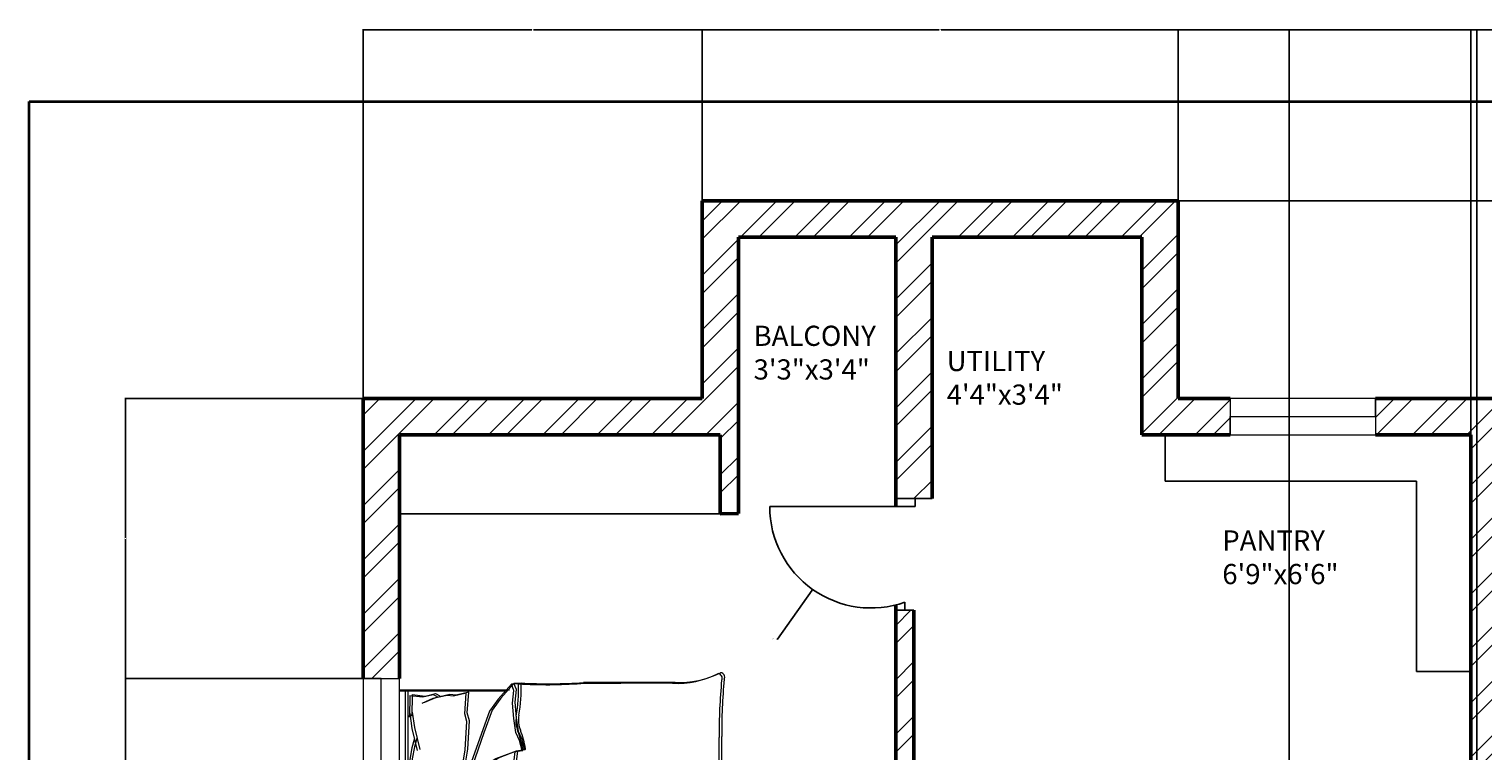
# Model space of a CAD drawing. Units: inches. Extents: x 1896 to 2572, y 1528 to 2474.
# Tile 8 of 10: x 1896 to 2256, y 2295 to 2474. Entities that reach past the tile are written whole.
import ezdxf

# ---------------------------------------------------------------- set-up
doc = ezdxf.new("R2010")
doc.units = ezdxf.units.IN
for name, color, linetype, lineweight in [('A-ANNO-DIMS', 2, 'Continuous', 18), ('A-ANNO-TTLB', 7, 'Continuous', 35), ('A-AREA-IDEN', 7, 'Continuous', 18), ('A-DOOR', 11, 'Continuous', 25), ('A-FLOR-CASE', 7, 'Continuous', 25), ('A-FURN', 8, 'Continuous', 18), ('A-GLAZ', 131, 'Continuous', 20), ('A-WALL', 7, 'Continuous', 50)]:
    doc.layers.add(name, color=color, linetype=linetype, lineweight=lineweight)
doc.layers.add('A-WALL-PATT', color=215, linetype='Continuous', lineweight=13, true_color=0xa953a0)
doc.styles.get("Standard").update_dxf_attribs({"font": 'arial.ttf'})
doc.dimstyles.get("Standard").update_dxf_attribs({"dimtxt": 0.18, "dimasz": 0.18, "dimexe": 0.18, "dimexo": 0.0625, "dimgap": 0.09, "dimtad": 0, "dimtih": 1, "dimtoh": 1, "dimdec": 4, "dimzin": 0, "dimdsep": 46, "dimtxsty": 'Standard', "dimcen": 0.09, "dimadec": 0, "dimazin": 0, "dimtfac": 1, "dimtdec": 4, "dimtofl": 0, "dimtmove": 0, "dimatfit": 3, "dimfxl": 1, "dimtolj": 1, "dimtzin": 0, "dimarcsym": 0})

# ---------------------------------------------------------------- blocks, each defined once
blk = doc.blocks.new('BED-DOUBLE')
for p, q in [((3.47, 63.33), (3.47, 81.44)), ((3.47, 63.33), (3.47, 81.44)), ((3.47, 81.44), (51.49, 81.44)), ((3.47, 79.91), (51.27, 79.91)), ((3.47, 79.91), (51.26, 79.91)), ((3.7, 62.69), (3.7, 80.8)), ((3.7, 62.69), (3.7, 80.8)), ((3.7, 79.27), (51.49, 79.27)), ((3.7, 79.27), (51.49, 79.27)), ((24.54, 78.99), (25.98, 79.57)), ((24.54, 78.99), (25.98, 79.57)), ((25.98, 79.57), (26.56, 74.22)), ((25.98, 79.57), (26.56, 74.22)), ((51.26, 81.44), (51.26, 54.83)), ((51.27, 81.44), (51.27, 54.83)), ((51.49, 81.44), (51.49, 80.8)), ((51.49, 80.8), (51.49, 54.19)), ((51.49, 80.8), (51.49, 54.19)), ((3.89, 78.13), (4.47, 74.95)), ((3.89, 78.13), (4.47, 74.95)), ((3.9, 78.11), (8.18, 78.43)), ((3.9, 78.11), (8.18, 78.43)), ((4.12, 77.49), (4.7, 74.31)), ((4.12, 77.49), (4.7, 74.31)), ((4.13, 77.47), (8.41, 77.8)), ((4.13, 77.47), (8.41, 77.8)), ((8.18, 78.43), (8.28, 78.42)), ((8.18, 78.43), (8.28, 78.42)), ((8.28, 78.42), (12.11, 78.13)), ((8.28, 78.42), (12.11, 78.13)), ((8.41, 77.8), (8.51, 77.78)), ((8.41, 77.8), (8.51, 77.78)), ((8.51, 77.78), (12.34, 77.49)), ((8.51, 77.78), (12.34, 77.49)), ((12.11, 78.13), (17.6, 77.12)), ((12.11, 78.13), (17.6, 77.12)), ((12.34, 77.49), (17.83, 76.48)), ((12.34, 77.49), (17.83, 76.48)), ((14.85, 77.69), (16.88, 78.42)), ((14.85, 77.69), (16.88, 78.42)), ((15.08, 77.05), (17.11, 77.78)), ((15.08, 77.05), (17.11, 77.78)), ((16.88, 78.42), (19.77, 79.14)), ((16.88, 78.42), (19.77, 79.14)), ((17.11, 77.78), (20, 78.5)), ((17.11, 77.78), (20, 78.5)), ((19.77, 79.14), (20.09, 79.14)), ((19.77, 79.14), (20.09, 79.14)), ((20, 78.5), (20.32, 78.5)), ((20, 78.5), (20.32, 78.5)), ((20.09, 79.14), (24.54, 78.99)), ((20.09, 79.14), (24.54, 78.99)), ((20.32, 78.5), (24.77, 78.36)), ((20.32, 78.5), (24.76, 78.36)), ((24.76, 78.36), (26.21, 78.93)), ((24.77, 78.36), (26.21, 78.93)), ((26.21, 78.93), (26.79, 73.58)), ((26.21, 78.93), (26.79, 73.58)), ((27.98, 78.95), (27.73, 73.58)), ((27.98, 78.95), (27.73, 73.58)), ((28.21, 78.31), (27.96, 72.94)), ((28.2, 78.31), (27.96, 72.94)), ((29.46, 78.46), (27.98, 78.95)), ((29.46, 78.46), (27.98, 78.95)), ((29.68, 77.83), (28.2, 78.31)), ((29.68, 77.83), (28.21, 78.31)), ((33.88, 78.89), (29.46, 78.46)), ((33.88, 78.89), (29.46, 78.46)), ((34.11, 78.25), (29.68, 77.83)), ((34.11, 78.25), (29.68, 77.83)), ((34.2, 78.91), (33.88, 78.89)), ((34.2, 78.91), (33.88, 78.89)), ((34.43, 78.27), (34.11, 78.25)), ((34.43, 78.27), (34.11, 78.25)), ((37.14, 78.37), (34.2, 78.91)), ((37.13, 78.37), (34.2, 78.91)), ((37.36, 77.73), (34.43, 78.27)), ((37.36, 77.73), (34.43, 78.27)), ((41.91, 78.37), (36.49, 77.02)), ((41.91, 78.37), (36.49, 77.02)), ((42.14, 77.73), (36.72, 76.38)), ((42.14, 77.73), (36.72, 76.38)), ((39.2, 77.77), (37.13, 78.37)), ((39.2, 77.77), (37.14, 78.37)), ((39.43, 77.13), (37.36, 77.73)), ((39.43, 77.13), (37.36, 77.73)), ((45.71, 78.9), (41.91, 78.37)), ((45.71, 78.9), (41.91, 78.37)), ((45.94, 78.26), (42.14, 77.73)), ((45.94, 78.26), (42.14, 77.73)), ((50.11, 78.89), (44.71, 78.98)), ((44.71, 78.98), (45.71, 78.9)), ((50.11, 78.89), (44.71, 78.98)), ((44.71, 78.98), (45.71, 78.9)), ((50.34, 78.25), (44.94, 78.34)), ((44.94, 78.34), (45.94, 78.26)), ((50.34, 78.25), (44.94, 78.34)), ((44.94, 78.34), (45.94, 78.26)), ((49.31, 73.19), (48.13, 75.87)), ((49.31, 73.19), (48.13, 75.87)), ((50.11, 78.89), (49.73, 75.68)), ((50.11, 78.89), (49.73, 75.68)), ((49.73, 75.68), (50.33, 73.11)), ((49.73, 75.68), (50.33, 73.11)), ((50.34, 78.25), (49.96, 75.04)), ((50.34, 78.25), (49.96, 75.04)), ((4.47, 74.95), (4.04, 72.34)), ((4.47, 74.95), (4.04, 72.34)), ((4.04, 72.34), (4.62, 71.33)), ((4.04, 72.34), (4.62, 71.33)), ((4.7, 74.31), (4.27, 71.7)), ((4.7, 74.31), (4.27, 71.7)), ((4.47, 68.87), (5.05, 72.49)), ((4.47, 68.87), (5.05, 72.49)), ((5.05, 72.49), (6.06, 75.24)), ((5.05, 72.49), (6.06, 75.24)), ((5.28, 71.85), (6.29, 74.6)), ((5.28, 71.85), (6.29, 74.6)), ((26.56, 74.22), (27.14, 71.04)), ((26.56, 74.22), (27.14, 71.04)), ((26.79, 73.58), (27.37, 70.4)), ((26.79, 73.58), (27.37, 70.4)), ((27.73, 73.58), (27.35, 70.37)), ((27.73, 73.58), (27.35, 70.37)), ((27.96, 72.94), (27.58, 69.73)), ((27.96, 72.94), (27.58, 69.73)), ((49.54, 72.55), (48.36, 75.23)), ((49.54, 72.55), (48.36, 75.23)), ((50.11, 69.61), (49.31, 73.19)), ((50.11, 69.61), (49.31, 73.19)), ((50.34, 68.98), (49.54, 72.55)), ((50.34, 68.98), (49.54, 72.55)), ((50.33, 73.11), (49.81, 72.06)), ((50.33, 73.11), (49.81, 72.06)), ((49.96, 75.04), (50.56, 72.47)), ((49.96, 75.04), (50.56, 72.47)), ((50.56, 72.47), (50.04, 71.42)), ((50.56, 72.47), (50.04, 71.42)), ((4.27, 71.7), (4.85, 70.69)), ((4.27, 71.7), (4.85, 70.69)), ((4.76, 67.28), (4.47, 68.87)), ((4.76, 67.28), (4.47, 68.87)), ((4.7, 68.23), (5.28, 71.85)), ((4.7, 68.23), (5.28, 71.85)), ((27.14, 69.74), (26.56, 67.86)), ((27.14, 69.74), (26.56, 67.86)), ((27.37, 69.1), (26.79, 67.22)), ((27.37, 69.1), (26.79, 67.22)), ((27.14, 71.04), (27.14, 69.74)), ((27.14, 71.04), (27.14, 69.74)), ((27.35, 70.37), (27.44, 69.07)), ((27.35, 70.37), (27.44, 69.07)), ((27.37, 70.4), (27.37, 69.1)), ((27.37, 70.4), (27.37, 69.1)), ((27.44, 69.07), (28.13, 67.23)), ((27.44, 69.07), (28.13, 67.23)), ((27.58, 69.73), (27.66, 68.43)), ((27.58, 69.73), (27.66, 68.43)), ((49.92, 68.01), (50.11, 69.61)), ((49.92, 68.01), (50.11, 69.61)), ((50.15, 67.37), (50.34, 68.98)), ((50.15, 67.37), (50.34, 68.98)), ((4.18, 64.1), (4.76, 67.28)), ((4.18, 64.1), (4.76, 67.28)), ((4.41, 63.46), (4.99, 66.64)), ((4.41, 63.46), (4.99, 66.64)), ((4.99, 66.64), (4.7, 68.23)), ((4.99, 66.64), (4.7, 68.23)), ((6.38, 65.81), (10.41, 65.15)), ((6.38, 65.81), (10.41, 65.15)), ((6.61, 65.18), (10.64, 64.51)), ((6.61, 65.18), (10.64, 64.51)), ((10.41, 65.15), (9.28, 64.83)), ((10.41, 65.15), (9.28, 64.83)), ((10.41, 65.15), (17.42, 64.72)), ((10.41, 65.15), (17.42, 64.72)), ((17.42, 64.72), (19.38, 65.27)), ((17.42, 64.72), (19.38, 65.27)), ((19.38, 65.27), (24.52, 64.87)), ((19.38, 65.27), (24.52, 64.87)), ((24.1, 65.18), (20.96, 66.27)), ((24.1, 65.18), (20.96, 66.27)), ((24.33, 64.54), (21.19, 65.63)), ((24.33, 64.54), (21.19, 65.63)), ((26.56, 65.18), (24.1, 65.18)), ((26.56, 65.18), (24.1, 65.18)), ((26.56, 67.86), (26.56, 65.18)), ((26.56, 67.86), (26.56, 65.18)), ((26.79, 67.22), (26.79, 64.54)), ((26.79, 67.22), (26.79, 64.54)), ((27.66, 68.43), (28.36, 66.59)), ((27.66, 68.43), (28.36, 66.59)), ((28.13, 67.23), (28.3, 64.55)), ((28.13, 67.23), (28.3, 64.55)), ((28.36, 66.59), (28.53, 63.91)), ((28.36, 66.59), (28.53, 63.91)), ((30.75, 64.7), (33.82, 65.99)), ((30.75, 64.7), (33.82, 65.99)), ((30.98, 64.06), (34.05, 65.35)), ((30.98, 64.06), (34.05, 65.35)), ((32.56, 65.81), (36.6, 65.15)), ((32.56, 65.81), (36.6, 65.15)), ((32.79, 65.18), (36.82, 64.51)), ((32.79, 65.18), (36.82, 64.51)), ((36.6, 65.15), (43.61, 64.72)), ((36.6, 65.15), (43.61, 64.72)), ((43.61, 64.72), (45.57, 65.27)), ((43.61, 64.72), (45.57, 65.27)), ((45.57, 65.27), (50.7, 64.87)), ((45.57, 65.27), (50.7, 64.87)), ((50.7, 64.87), (49.92, 68.01)), ((50.7, 64.87), (49.92, 68.01)), ((50.93, 64.23), (50.15, 67.37)), ((50.93, 64.23), (50.15, 67.37)), ((9.28, 64.83), (4.18, 64.1)), ((9.28, 64.83), (4.18, 64.1)), ((9.51, 64.19), (4.41, 63.46)), ((9.51, 64.19), (4.41, 63.46)), ((10.64, 64.51), (9.51, 64.19)), ((10.64, 64.51), (9.51, 64.19)), ((10.64, 64.51), (17.65, 64.08)), ((10.64, 64.51), (17.65, 64.08)), ((17.65, 64.08), (19.61, 64.63)), ((17.65, 64.08), (19.61, 64.63)), ((19.61, 64.63), (24.74, 64.23)), ((19.61, 64.63), (24.74, 64.23)), ((26.79, 64.54), (24.33, 64.54)), ((26.79, 64.54), (24.33, 64.54)), ((28.3, 64.55), (30.75, 64.7)), ((28.3, 64.55), (30.75, 64.7)), ((28.53, 63.91), (30.98, 64.06)), ((28.53, 63.91), (30.98, 64.06)), ((30.26, 64.06), (34.45, 57.57)), ((30.26, 64.06), (34.45, 57.57)), ((30.49, 63.42), (34.68, 56.93)), ((30.49, 63.42), (34.68, 56.93)), ((40.64, 61.13), (32.31, 64.06)), ((40.64, 61.13), (32.31, 64.06)), ((40.87, 60.49), (32.53, 63.42)), ((40.87, 60.49), (32.53, 63.42)), ((36.82, 64.51), (43.83, 64.08)), ((36.82, 64.51), (43.83, 64.08)), ((43.83, 64.08), (45.79, 64.63)), ((43.83, 64.08), (45.79, 64.63)), ((45.79, 64.63), (50.93, 64.23)), ((45.79, 64.63), (50.93, 64.23)), ((46.22, 59.11), (40.64, 61.13)), ((46.22, 59.11), (40.64, 61.13)), ((46.45, 58.48), (40.87, 60.49)), ((46.45, 58.48), (40.87, 60.49)), ((49.16, 56.95), (46.22, 59.11)), ((49.16, 56.95), (46.22, 59.11)), ((49.39, 56.31), (46.45, 58.48)), ((49.39, 56.31), (46.45, 58.48)), ((34.45, 57.57), (36.15, 53.08)), ((34.45, 57.57), (36.15, 53.08)), ((34.68, 56.93), (36.38, 52.44)), ((34.68, 56.93), (36.38, 52.44)), ((52.87, 53.7), (49.16, 56.95)), ((52.87, 53.7), (49.16, 56.95)), ((53.1, 53.06), (49.39, 56.31)), ((53.1, 53.06), (49.39, 56.31)), ((36.15, 53.08), (36.46, 51.07)), ((36.15, 53.08), (36.46, 51.07)), ((36.38, 52.44), (36.69, 50.43)), ((36.38, 52.44), (36.69, 50.43)), ((36.46, 51.07), (38.94, 51.69)), ((36.46, 51.07), (38.94, 51.69)), ((36.69, 50.43), (39.17, 51.05)), ((36.69, 50.43), (39.17, 51.05)), ((38.94, 51.69), (40.95, 52.61)), ((38.94, 51.69), (40.95, 52.61)), ((39.17, 51.05), (41.18, 51.97)), ((39.17, 51.05), (41.18, 51.97)), ((40.95, 52.61), (44.36, 53.08)), ((40.95, 52.61), (44.36, 53.08)), ((41.18, 51.97), (44.59, 52.44)), ((41.18, 51.97), (44.59, 52.44)), ((44.36, 53.08), (48.23, 53.39)), ((44.36, 53.08), (48.23, 53.39)), ((44.59, 52.44), (48.46, 52.75)), ((44.59, 52.44), (48.46, 52.75)), ((48.23, 53.39), (51.33, 53.08)), ((48.23, 53.39), (51.33, 53.08)), ((48.46, 52.75), (51.56, 52.44)), ((48.46, 52.75), (51.56, 52.44)), ((51.33, 53.08), (52.87, 53.7)), ((51.33, 53.08), (52.87, 53.7)), ((51.56, 52.44), (53.1, 53.06)), ((51.56, 52.44), (53.1, 53.06)), ((52.95, 51.95), (52.87, 53.7, 3.87)), ((52.95, 51.95), (52.87, 53.7, 3.87)), ((53.18, 51.31), (53.1, 53.06, 3.87)), ((53.17, 51.31), (53.1, 53.06, 3.87)), ((15.06, 2.2), (39.68, 2.2)), ((15.06, 2.2), (39.68, 2.2)), ((15.29, 1.56), (39.91, 1.56)), ((15.29, 1.56), (39.91, 1.56))]:
    blk.add_line(p, q)
for centre, radius, start, end in [((85.16, 61.35), 83.31, 178.7218, 185.604), ((85.16, 61.35), 83.31, 178.7218, 185.604), ((21.36, -100.61), 164.97, 86.0865, 96.7821), ((21.36, -100.61), 164.97, 86.0865, 96.7821), ((85.39, 60.71), 83.31, 178.7218, 185.604), ((85.39, 60.71), 83.31, 178.7218, 185.604), ((21.59, -101.25), 164.97, 86.0865, 96.7821), ((21.59, -101.25), 164.97, 86.0865, 96.7821), ((17.76, -74.87), 129.02, 81.7845, 96.9006), ((17.76, -74.87), 129.02, 81.7845, 96.9006), ((17.98, -75.51), 129.02, 81.7845, 96.9006), ((17.98, -75.51), 129.02, 81.7845, 96.9006), ((-167.31, 50.27), 170.11, 358.4762, 1.0082), ((-167.31, 50.27), 170.11, 358.4762, 1.0082), ((-167.08, 49.63), 170.11, 358.4762, 1.0082), ((-167.08, 49.63), 170.11, 358.4762, 1.0082), ((36.64, 51), 0.185, 160.2464, 271.1377), ((36.64, 51), 0.185, 160.2464, 271.1377), ((31.15, 79.96), 29.65, 280.6617, 289.8806), ((31.15, 79.96), 29.65, 280.6617, 289.8806), ((31.38, 79.32), 29.65, 280.6617, 289.8806), ((31.38, 79.32), 29.65, 280.6617, 289.8806), ((43.74, 46.38), 6.22, 78.6608, 113.7384), ((43.74, 46.38), 6.22, 78.6608, 113.7384), ((43.97, 45.74), 6.22, 78.6608, 113.7384), ((43.97, 45.74), 6.22, 78.6608, 113.7384), ((51.33, 88.1), 36.18, 259.8763, 272.5657), ((51.33, 88.1), 36.18, 259.8763, 272.5657), ((51.56, 87.46), 36.18, 259.8763, 272.5657), ((51.56, 87.46), 36.18, 259.8763, 272.5657), ((182.27, 45.13), 129.5, 176.9791, 183.8365), ((182.27, 45.13), 129.5, 176.9791, 183.8365), ((182.49, 44.49), 129.5, 176.9791, 183.8365), ((182.49, 44.49), 129.5, 176.9791, 183.8365), ((36.86, 50.36), 0.185, 160.2464, 271.1377), ((36.86, 50.36), 0.185, 160.2464, 271.1377), ((484.82, 30.83), 482.31, 178.2277, 181.7185), ((484.82, 30.83), 482.31, 178.2277, 181.7185), ((485.05, 30.19), 482.31, 178.2277, 181.7185), ((485.05, 30.19), 482.31, 178.2277, 181.7185), ((-4508.74, 13.62), 4561.86, 0.00217, 0.28689), ((-4508.74, 13.62), 4561.86, 0.00217, 0.28689), ((-4508.52, 12.98), 4561.86, 0.00217, 0.28689), ((-4508.52, 12.98), 4561.86, 0.00217, 0.28689), ((-26.9, 16.93), 29.63, 346.0648, 358.9113), ((-26.9, 16.93), 29.63, 346.0648, 358.9113), ((-26.67, 16.29), 29.63, 346.0648, 358.9113), ((-26.67, 16.29), 29.63, 346.0648, 358.9113), ((76.16, 12.78), 23.07, 177.4714, 206.4681), ((76.16, 12.78), 23.07, 177.4714, 206.4681), ((76.39, 12.14), 23.07, 177.4714, 206.4681), ((76.39, 12.14), 23.07, 177.4714, 206.4681), ((-21.66, 11.17), 23.56, 337.9751, 356.652), ((-21.66, 11.17), 23.56, 337.9751, 356.652), ((-21.43, 10.53), 23.56, 337.9751, 356.652), ((-21.43, 10.53), 23.56, 337.9751, 356.652), ((-17.22, 105.16), 106.46, 283.3832, 287.7053), ((-17.22, 105.16), 106.46, 283.3832, 287.7053), ((1.09, 1.73), 1.09, 146.1736, 293.4781), ((1.09, 1.73), 1.09, 146.1736, 293.4781), ((1.32, 1.09), 1.09, 146.1736, 293.4781), ((1.32, 1.09), 1.09, 146.1736, 293.4781), ((21.43, -119.39), 121.76, 92.9958, 99.4091), ((21.43, -119.39), 121.76, 92.9958, 99.4091), ((21.65, -120.03), 121.76, 92.9958, 99.4091), ((21.65, -120.03), 121.76, 92.9958, 99.4091), ((-16.99, 104.52), 106.46, 283.3832, 287.7053), ((-16.99, 104.52), 106.46, 283.3832, 287.7053), ((41.15, -130.83), 133.04, 84.4998, 90.6351), ((41.15, -130.83), 133.04, 84.4998, 90.6351), ((41.38, -131.47), 133.04, 84.4998, 90.6351), ((41.38, -131.47), 133.04, 84.4998, 90.6351), ((54.41, 2.57), 1.1, 242.6588, 356.02), ((54.41, 2.57), 1.1, 242.6588, 356.02), ((54.64, 1.93), 1.1, 242.6588, 356.02), ((54.64, 1.93), 1.1, 242.6588, 356.02)]:
    blk.add_arc(centre, radius, start, end)
blk = doc.blocks.new('WIN-36IN')
for p, q in [((0, 36), (9, 36)), ((0, 0), (0, 36)), ((9, 36), (4.5, 36)), ((4.5, 36), (4.5, 0)), ((9, 36), (9, 0)), ((4.5, 0), (0, 0)), ((0, 0), (9, 0))]:
    blk.add_line(p, q)
blk = doc.blocks.new('WIN-60IN')
for p, q in [((4.5, 60), (0, 60)), ((0, 60), (9, 60)), ((0, 60), (0, 0)), ((4.5, 0), (4.5, 60)), ((9, 0), (9, 60)), ((0, 0), (9, 0)), ((9, 0), (4.5, 0))]:
    blk.add_line(p, q)
blk = doc.blocks.new('*D20')
at = {"layer": 'A-ANNO-DIMS', "color": 0, "lineweight": -2, "transparency": 16777216}
for p, q in [((2180.68, 2431.4), (2511.65, 2431.4)), ((2511.47, 2431.22), (2511.47, 2049.83)), ((2511.47, 1668.08), (2511.47, 2049.47)), ((2452.68, 1667.9), (2511.65, 1667.9))]:
    blk.add_line(p, q, dxfattribs=at)
at = {"layer": 'A-ANNO-DIMS', "color": 0, "transparency": 16777216}
for points in [[(2511.44, 2431.22), (2511.5, 2431.22), (2511.47, 2431.4)], [(2511.44, 1668.08), (2511.5, 1668.08), (2511.47, 1667.9)]]:
    blk.add_solid(points, dxfattribs=at)
at = {"layer": 'Defpoints', "color": 0, "transparency": 16777216}
for p in [(2180.62, 2431.4), (2511.47, 2431.4), (2452.62, 1667.9)]:
    blk.add_point(p, dxfattribs=at)
at = {"layer": 'A-ANNO-DIMS', "color": 0, "transparency": 16777216, "insert": (2511.47, 2049.65), "char_height": 0.18, "attachment_point": 5}
blk.add_mtext('\\A1;763.5', dxfattribs=at)
blk = doc.blocks.new('*D21')
at = {"layer": 'A-ANNO-DIMS', "color": 0, "lineweight": -2, "transparency": 16777216}
for p, q in [((1978.62, 2382.46), (1978.62, 2473.93)), ((1978.8, 2473.75), (2020.4, 2473.75)), ((2062.44, 2473.75), (2020.84, 2473.75)), ((2062.62, 2431.46), (2062.62, 2473.93))]:
    blk.add_line(p, q, dxfattribs=at)
at = {"layer": 'A-ANNO-DIMS', "color": 0, "transparency": 16777216}
for points in [[(1978.8, 2473.78), (1978.8, 2473.72), (1978.62, 2473.75)], [(2062.44, 2473.78), (2062.44, 2473.72), (2062.62, 2473.75)]]:
    blk.add_solid(points, dxfattribs=at)
at = {"layer": 'Defpoints', "color": 0, "transparency": 16777216}
for p in [(2062.62, 2473.75), (2062.62, 2431.4), (1978.62, 2382.4)]:
    blk.add_point(p, dxfattribs=at)
at = {"layer": 'A-ANNO-DIMS', "color": 0, "transparency": 16777216, "insert": (2020.62, 2473.75), "char_height": 0.18, "attachment_point": 5}
blk.add_mtext('\\A1;84', dxfattribs=at)
blk = doc.blocks.new('*D22')
at = {"layer": 'A-ANNO-DIMS', "color": 0, "lineweight": -2, "transparency": 16777216}
for p, q in [((2062.62, 2431.46), (2062.62, 2473.93)), ((2062.8, 2473.75), (2121.34, 2473.75)), ((2180.44, 2473.75), (2121.9, 2473.75)), ((2180.62, 2431.46), (2180.62, 2473.93))]:
    blk.add_line(p, q, dxfattribs=at)
at = {"layer": 'A-ANNO-DIMS', "color": 0, "transparency": 16777216}
for points in [[(2062.8, 2473.78), (2062.8, 2473.72), (2062.62, 2473.75)], [(2180.44, 2473.78), (2180.44, 2473.72), (2180.62, 2473.75)]]:
    blk.add_solid(points, dxfattribs=at)
at = {"layer": 'Defpoints', "color": 0, "transparency": 16777216}
for p in [(2180.62, 2473.75), (2062.62, 2431.4), (2180.62, 2431.4)]:
    blk.add_point(p, dxfattribs=at)
at = {"layer": 'A-ANNO-DIMS', "color": 0, "transparency": 16777216, "insert": (2121.62, 2473.75), "char_height": 0.18, "attachment_point": 5}
blk.add_mtext('\\A1;118', dxfattribs=at)
blk = doc.blocks.new('*D23')
at = {"layer": 'A-ANNO-DIMS', "color": 0, "lineweight": -2, "transparency": 16777216}
for p, q in [((2180.62, 2431.46), (2180.62, 2473.93)), ((2180.8, 2473.75), (2216.55, 2473.75)), ((2252.94, 2473.75), (2217.2, 2473.75)), ((2253.12, 2373.46), (2253.12, 2473.93))]:
    blk.add_line(p, q, dxfattribs=at)
at = {"layer": 'A-ANNO-DIMS', "color": 0, "transparency": 16777216}
for points in [[(2180.8, 2473.78), (2180.8, 2473.72), (2180.62, 2473.75)], [(2252.94, 2473.78), (2252.94, 2473.72), (2253.12, 2473.75)]]:
    blk.add_solid(points, dxfattribs=at)
at = {"layer": 'Defpoints', "color": 0, "transparency": 16777216}
for p in [(2253.12, 2473.75), (2180.62, 2431.4), (2253.12, 2373.4)]:
    blk.add_point(p, dxfattribs=at)
at = {"layer": 'A-ANNO-DIMS', "color": 0, "transparency": 16777216, "insert": (2216.87, 2473.75), "char_height": 0.18, "attachment_point": 5}
blk.add_mtext('\\A1;72.5', dxfattribs=at)
blk = doc.blocks.new('*D24')
at = {"layer": 'A-ANNO-DIMS', "color": 0, "lineweight": -2, "transparency": 16777216}
for p, q in [((2253.12, 2373.46), (2253.12, 2473.93)), ((2253.3, 2473.75), (2352.49, 2473.75)), ((2452.44, 2473.75), (2353.26, 2473.75)), ((2452.62, 2382.46), (2452.62, 2473.93))]:
    blk.add_line(p, q, dxfattribs=at)
at = {"layer": 'A-ANNO-DIMS', "color": 0, "transparency": 16777216}
for points in [[(2253.3, 2473.78), (2253.3, 2473.72), (2253.12, 2473.75)], [(2452.44, 2473.78), (2452.44, 2473.72), (2452.62, 2473.75)]]:
    blk.add_solid(points, dxfattribs=at)
at = {"layer": 'Defpoints', "color": 0, "transparency": 16777216}
for p in [(2452.62, 2473.75), (2452.62, 2382.4), (2253.12, 2373.4)]:
    blk.add_point(p, dxfattribs=at)
at = {"layer": 'A-ANNO-DIMS', "color": 0, "transparency": 16777216, "insert": (2352.87, 2473.75), "char_height": 0.18, "attachment_point": 5}
blk.add_mtext('\\A1;199.5', dxfattribs=at)
blk = doc.blocks.new('*D25')
at = {"layer": 'A-ANNO-DIMS', "color": 0, "lineweight": -2, "transparency": 16777216}
for p, q in [((1978.56, 2382.4), (1919.59, 2382.4)), ((1919.77, 2382.22), (1919.77, 2347.9)), ((1919.77, 2313.21), (1919.77, 2347.53)), ((1978.56, 2313.03), (1919.59, 2313.03))]:
    blk.add_line(p, q, dxfattribs=at)
at = {"layer": 'A-ANNO-DIMS', "color": 0, "transparency": 16777216}
for points in [[(1919.74, 2382.22), (1919.8, 2382.22), (1919.77, 2382.4)], [(1919.74, 2313.21), (1919.8, 2313.21), (1919.77, 2313.03)]]:
    blk.add_solid(points, dxfattribs=at)
at = {"layer": 'Defpoints', "color": 0, "transparency": 16777216}
for p in [(1978.62, 2382.4), (1919.77, 2313.03), (1978.62, 2313.03)]:
    blk.add_point(p, dxfattribs=at)
at = {"layer": 'A-ANNO-DIMS', "color": 0, "transparency": 16777216, "insert": (1919.77, 2347.72), "char_height": 0.18, "attachment_point": 5}
blk.add_mtext('\\A1;69.36', dxfattribs=at)
blk = doc.blocks.new('*D26')
at = {"layer": 'A-ANNO-DIMS', "color": 0, "lineweight": -2, "transparency": 16777216}
for p, q in [((1978.56, 2313.03), (1919.59, 2313.03)), ((1919.77, 2312.85), (1919.77, 2244.65)), ((1919.77, 2176.08), (1919.77, 2244.28)), ((1987.56, 2175.9), (1919.59, 2175.9))]:
    blk.add_line(p, q, dxfattribs=at)
at = {"layer": 'A-ANNO-DIMS', "color": 0, "transparency": 16777216}
for points in [[(1919.74, 2312.85), (1919.8, 2312.85), (1919.77, 2313.03)], [(1919.74, 2176.08), (1919.8, 2176.08), (1919.77, 2175.9)]]:
    blk.add_solid(points, dxfattribs=at)
at = {"layer": 'Defpoints', "color": 0, "transparency": 16777216}
for p in [(1978.62, 2313.03), (1919.77, 2175.9), (1987.62, 2175.9)]:
    blk.add_point(p, dxfattribs=at)
at = {"layer": 'A-ANNO-DIMS', "color": 0, "transparency": 16777216, "insert": (1919.77, 2244.47), "char_height": 0.18, "attachment_point": 5}
blk.add_mtext('\\A1;137.14', dxfattribs=at)
blk = doc.blocks.new('*D34')
at = {"layer": 'A-ANNO-DIMS', "color": 0, "lineweight": -2, "transparency": 16777216}
for p, q in [((2208.12, 1889.96), (2208.12, 2473.93)), ((2208.3, 2473.75), (2231.04, 2473.75)), ((2254.44, 2473.75), (2231.7, 2473.75)), ((2254.62, 1889.96), (2254.62, 2473.93))]:
    blk.add_line(p, q, dxfattribs=at)
at = {"layer": 'A-ANNO-DIMS', "color": 0, "transparency": 16777216}
for points in [[(2208.3, 2473.78), (2208.3, 2473.72), (2208.12, 2473.75)], [(2254.44, 2473.78), (2254.44, 2473.72), (2254.62, 2473.75)]]:
    blk.add_solid(points, dxfattribs=at)
at = {"layer": 'Defpoints', "color": 0, "transparency": 16777216}
for p in [(2254.62, 2473.75), (2208.12, 1889.9), (2254.62, 1889.9)]:
    blk.add_point(p, dxfattribs=at)
at = {"layer": 'A-ANNO-DIMS', "color": 0, "transparency": 16777216, "insert": (2231.37, 2473.75), "char_height": 0.18, "attachment_point": 5}
blk.add_mtext('\\A1;46.5', dxfattribs=at)
blk = doc.blocks.new('*D45')
at = {"layer": 'A-ANNO-DIMS', "color": 0, "lineweight": -2, "transparency": 16777216}
for p, q in [((2104.42, 2355.6), (2104.6, 2355.6)), ((2104.51, 2355.51), (2104.51, 2355.69)), ((2081.31, 2322.77), (2089.91, 2334.93)), ((2081.13, 2322.77), (2081.31, 2322.77))]:
    blk.add_line(p, q, dxfattribs=at)
at = {"layer": 'A-ANNO-DIMS', "color": 0, "transparency": 16777216}
blk.add_solid([(2089.88, 2334.95), (2089.93, 2334.91), (2090.01, 2335.08)], dxfattribs=at)
at = {"layer": 'Defpoints', "color": 0, "transparency": 16777216}
for p in [(2104.51, 2355.6), (2090.01, 2335.08)]:
    blk.add_point(p, dxfattribs=at)
at = {"layer": 'A-ANNO-DIMS', "color": 0, "transparency": 16777216, "insert": (2080.58, 2322.77), "char_height": 0.18, "attachment_point": 5}
blk.add_mtext('\\A1;R25.123', dxfattribs=at)

msp = doc.modelspace()

# ---------------------------------------------------------------- hatches: boundary and pattern name
at = {"layer": 'A-WALL-PATT'}
h = msp.add_hatch(dxfattribs=at)
h.set_pattern_fill('ANSI32', color=256)
h.paths.add_polyline_path([(2071.6224, 2382.3979), (2071.6224, 2422.3979), (2110.6224, 2422.3979), (2110.6224, 2382.3979), (2110.6224, 2357.5961), (2119.6224, 2357.5961), (2119.6224, 2422.3979), (2171.6224, 2422.3979), (2171.6224, 2373.3979), (2193.5093, 2373.3979), (2193.5093, 2377.8979), (2193.5093, 2382.3979), (2180.6224, 2382.3979), (2180.6224, 2431.3979), (2171.6224, 2431.3979), (2119.6224, 2431.3979), (2110.6224, 2431.3979), (2062.6224, 2431.3979), (2062.6224, 2422.3979), (2062.6224, 2382.3979), (1978.6224, 2382.3979), (1978.6224, 2313.0337), (1987.6224, 2313.0337), (1987.6224, 2373.3979), (2062.6224, 2373.3979), (2067.1224, 2373.3979), (2067.1224, 2353.7982), (2071.6224, 2353.8883)])
h.paths.add_polyline_path([(2287.4624, 2382.3979), (2229.5093, 2382.3979), (2229.5093, 2373.3979), (2253.1224, 2373.3979), (2253.1224, 2175.8979), (2247.1039, 2175.8979), (2247.1039, 2166.8979), (2253.1224, 2166.8979), (2253.1224, 2150.8283), (2262.1224, 2150.8283), (2262.1224, 2166.8979), (2262.1224, 2236.8979), (2349.0731, 2236.8979), (2349.0731, 2239.1479), (2349.0731, 2241.3979), (2262.1224, 2241.3979), (2262.1224, 2373.3979), (2287.4624, 2373.3979)])
h.paths.add_polyline_path([(2452.6224, 2382.3979), (2347.4624, 2382.3979), (2347.4624, 2373.3979), (2382.1224, 2373.3979), (2382.1224, 2334.0335), (2386.6224, 2334.0335), (2386.6224, 2373.3979), (2443.6224, 2373.3979), (2443.6224, 2316.2056), (2452.6224, 2316.2056)])
h.paths.add_polyline_path([(2452.6224, 2292.2056), (2448.1224, 2292.2056), (2443.6224, 2292.2056), (2443.6224, 2292.0047), (2443.6224, 2280.9372), (2443.6224, 2268.3979), (2386.6224, 2268.3979), (2386.6224, 2312.4044), (2384.3724, 2312.4044), (2382.1224, 2312.4044), (2382.1224, 2241.3979), (2379.1336, 2241.3979), (2379.1336, 2236.8979), (2386.6224, 2236.8979), (2386.6224, 2263.8979), (2443.6224, 2263.8979), (2443.6224, 2248.8449), (2452.6224, 2248.8449)])
h.paths.add_polyline_path([(2364.1285, 2116.8979), (2262.1224, 2116.8979), (2262.1224, 2120.5401), (2257.6224, 2120.5401), (2253.1224, 2120.5401), (2253.1224, 2107.8979), (2262.1224, 2107.8979), (2269.354, 2107.8979), (2269.354, 2094.0702), (2278.354, 2094.0702), (2278.354, 2107.8979), (2347.6224, 2107.8979), (2347.6224, 2039.8979), (2278.354, 2039.8979), (2278.354, 2054.7605), (2269.354, 2054.7605), (2269.354, 2030.8979), (2278.354, 2030.8979), (2443.6224, 2030.8979), (2443.6224, 2015.198), (2452.6224, 2015.198), (2452.6224, 2030.8979), (2464.6224, 2030.8979), (2469.1224, 2030.8979), (2469.1224, 2117.0352), (2452.6767, 2116.9466), (2452.6285, 2125.8979), (2452.6224, 2125.8979), (2452.6224, 2212.8449), (2443.6224, 2212.8449), (2443.6224, 2116.8979), (2385.832, 2116.8979), (2385.832, 2112.3979), (2385.832, 2107.8979), (2464.6224, 2107.8979), (2464.6224, 2039.8979), (2443.6224, 2039.8979), (2356.6224, 2039.8979), (2356.6224, 2107.8979), (2364.1285, 2107.8979)])
h.paths.add_polyline_path([(2452.6224, 1967.198), (2443.6224, 1967.198), (2443.6224, 1955.8979), (2259.1224, 1955.8979), (2254.6224, 1955.8979), (2254.6224, 1941.6358), (2263.6224, 1941.6358), (2263.6224, 1946.8979), (2379.1224, 1946.8979), (2379.1224, 1913.0204), (2383.6224, 1913.0204), (2383.6224, 1946.8979), (2443.6224, 1946.8979), (2443.6224, 1930.729), (2452.6224, 1930.729)])
h.paths.add_polyline_path([(2469.1224, 1871.8979), (2464.6224, 1871.8979), (2452.6224, 1871.8979), (2452.6224, 1894.729), (2443.6224, 1894.729), (2443.6224, 1871.8979), (2388.1304, 1871.8979), (2388.1304, 1867.3979), (2443.6224, 1867.3979), (2464.6224, 1867.3979), (2464.6224, 1817.8979), (2443.6224, 1817.8979), (2388.1304, 1817.8979), (2388.1304, 1815.6479), (2388.1304, 1813.3979), (2391.1224, 1813.3979), (2391.1224, 1747.8899), (2395.6224, 1747.8899), (2395.6224, 1813.3979), (2443.6224, 1813.3979), (2443.6224, 1781.4434), (2452.6224, 1781.4434), (2452.6224, 1813.3979), (2464.6224, 1813.3979), (2469.1224, 1813.3979)])
h.paths.add_polyline_path([(2263.6224, 1910.9737), (2259.1224, 1910.9737), (2254.6224, 1910.9737), (2254.6224, 1889.8979), (2251.2778, 1889.8979), (2251.2778, 1880.8979), (2254.6224, 1880.8979), (2254.6224, 1817.8979), (2254.6224, 1754.8979), (2254.6224, 1693.3979), (2254.6224, 1684.3979), (2254.6224, 1672.3979), (2200.6224, 1672.3979), (2200.6224, 1684.3979), (2200.6224, 1693.3979), (2200.6224, 1754.8979), (2196.1224, 1754.8979), (2196.1224, 1693.3979), (2150.0488, 1693.3979), (2150.0488, 1684.3979), (2196.1224, 1684.3979), (2196.1224, 1672.3979), (2196.1224, 1667.8979), (2254.6224, 1667.8979), (2259.1224, 1667.8979), (2259.1224, 1693.3979), (2259.1224, 1813.3979), (2353.6224, 1813.3979), (2353.6224, 1815.6479), (2353.6224, 1817.8979), (2263.6224, 1817.8979)])
h.paths.add_polyline_path([(2391.1224, 1693.3979), (2345.6981, 1693.3979), (2345.6981, 1684.3979), (2391.1224, 1684.3979)])
h.paths.add_polyline_path([(2285.6981, 1693.3979), (2259.1224, 1693.3979), (2259.1224, 1684.3979), (2285.6981, 1684.3979), (2285.6981, 1688.8979)], flags=17)
h.paths.add_polyline_path([(2452.6224, 1757.4434), (2448.1224, 1757.4434), (2443.6224, 1757.4434), (2443.6224, 1726.3979), (2395.6224, 1726.3979), (2395.6224, 1728.6572), (2393.3724, 1728.6572), (2391.1224, 1728.6572), (2391.1224, 1717.6723), (2395.6224, 1717.6723), (2395.6224, 1721.8979), (2443.6224, 1721.8979), (2443.6224, 1714.8), (2452.6224, 1714.8)])
h.paths.add_polyline_path([(2452.6224, 1684.3979), (2452.6224, 1690.8), (2443.6224, 1690.8), (2443.6224, 1679.8979), (2443.6224, 1672.3979), (2395.6224, 1672.3979), (2395.6224, 1695.6708), (2391.1224, 1695.5986), (2391.1224, 1672.3979), (2391.1224, 1667.8979), (2452.6224, 1667.8979)])
h.paths.add_polyline_path([(1987.6224, 1880.8979), (2068.6224, 1880.8979), (2125.6224, 1880.8979), (2125.6224, 1788.8466), (2130.1224, 1788.8466), (2130.1224, 1880.8979), (2216.1958, 1880.8979), (2216.1958, 1885.3979), (2216.1958, 1889.8979), (2208.1224, 1889.8979), (2208.1224, 1996.3717), (2203.6224, 1996.3717), (2199.1224, 1996.3717), (2199.1224, 1889.8979), (2073.1224, 1889.8979), (2073.1224, 1917.1874), (2068.6224, 1917.1874), (2068.6224, 1889.8979), (1987.6224, 1889.8979), (1987.6224, 1912.4976), (1978.6224, 1912.4976), (1978.6224, 1805.5193), (1987.6224, 1805.5193)])
h.paths.add_polyline_path([(2019.9303, 1754.8979), (1987.6224, 1754.8979), (1966.6224, 1754.8979), (1966.6224, 1801.0193), (1987.6224, 1801.0193), (1987.6224, 1805.5193), (1962.1224, 1805.5193), (1962.1224, 1750.3979), (1966.6224, 1750.3979), (1978.6224, 1750.3979), (1987.6224, 1750.3979), (2019.9303, 1750.3979)])
h.paths.add_polyline_path([(2135.5566, 1754.8979), (2130.1224, 1754.8979), (2130.1224, 1758.052), (2127.8724, 1758.052), (2125.6224, 1758.052), (2125.6224, 1754.8979), (2068.6224, 1754.8979), (2043.2292, 1754.8979), (2043.2292, 1750.3979), (2068.6224, 1750.3979), (2098.6224, 1750.3979), (2098.6224, 1693.3979), (2068.6224, 1693.3979), (1987.6224, 1693.3979), (1987.6224, 1707.3003), (1983.1224, 1707.3003), (1978.6224, 1707.3003), (1978.6224, 1684.3979), (2068.6224, 1684.3979), (2126.0488, 1684.3979), (2126.0488, 1688.8979), (2126.0488, 1693.3979), (2103.1224, 1693.3979), (2103.1224, 1750.3979), (2130.1224, 1750.3979), (2135.5566, 1750.3979)])
h.paths.add_polyline_path([(1987.6224, 1750.3979), (1978.6224, 1750.3979), (1978.6224, 1731.3003), (1987.6224, 1731.3003)], flags=0)
h.paths.add_polyline_path([(1987.6224, 1973.8979), (2068.6224, 1973.8979), (2073.1224, 1973.8979), (2073.1224, 1978.3979), (1971.1224, 1978.3979), (1971.1224, 2030.3979), (1978.6224, 2030.3979), (1987.6224, 2030.3979), (2104.9199, 2030.3979), (2104.9199, 2032.6479), (2104.9199, 2034.8979), (1987.6224, 2034.8979), (1971.1224, 2034.8979), (1971.1224, 2085.8979), (2003.6464, 2085.8979), (2003.6464, 2090.3979), (1987.6224, 2090.3979), (1987.6224, 2166.8979), (2115.1224, 2166.8979), (2137.6224, 2166.8979), (2137.6224, 2114.4229), (2142.1224, 2114.4229), (2142.1224, 2124.8979), (2153.5306, 2124.8979), (2153.5306, 2127.1479), (2153.5306, 2129.3979), (2142.1224, 2129.3979), (2142.1224, 2166.8979), (2199.1224, 2166.8979), (2199.1224, 2129.3979), (2177.5306, 2129.3979), (2177.5306, 2124.8979), (2199.1224, 2124.8979), (2199.1224, 2034.8979), (2142.1224, 2034.8979), (2142.1224, 2091.6671), (2139.8724, 2091.6671), (2137.6224, 2091.6671), (2137.6224, 2034.8979), (2133.8326, 2034.8979), (2133.8326, 2030.3979), (2137.6224, 2030.3979), (2142.1224, 2030.3979), (2199.1224, 2030.3979), (2199.1224, 2024.2654), (2208.1224, 2024.2654), (2208.1224, 2030.3979), (2208.1224, 2166.8979), (2214.5775, 2166.8979), (2214.5775, 2171.3979), (2214.5775, 2175.8979), (2115.1224, 2175.8979), (2115.1224, 2329.9154), (2112.4137, 2329.9154), (2110.6224, 2329.9154), (2110.6224, 2175.8979), (2082.1224, 2175.8979), (2082.1224, 2202.6443), (2079.8724, 2202.6443), (2077.6224, 2202.6443), (2077.6224, 2175.8979), (1987.6224, 2175.8979), (1987.6224, 2191.3531), (1983.1224, 2191.3531), (1978.6224, 2191.3531), (1978.6224, 2090.3979), (1966.6224, 2090.3979), (1966.6224, 2085.8979), (1966.6224, 2030.3979), (1966.6224, 1973.8979), (1978.6224, 1973.8979), (1978.6224, 1948.4976), (1983.1224, 1948.4976), (1987.6224, 1948.4976)])
h.paths.add_polyline_path([(1987.6224, 2253.0337), (1983.1224, 2253.0337), (1978.6224, 2253.0337), (1978.6224, 2215.3531), (1987.6224, 2215.3531), (1987.6224, 2224.8979), (2077.6224, 2224.8979), (2077.6224, 2221.9854), (2082.1224, 2221.9854), (2082.1224, 2229.3979), (1987.6224, 2229.3979)], flags=17)
h.paths.add_polyline_path([(2220.5047, 1978.7278), (2253.7278, 1978.7278), (2253.7278, 1997.3851), (2220.5047, 1997.3851)], flags=9)
h.paths.add_polyline_path([(2303.6746, 2064.9806), (2320.5334, 2064.9806), (2320.5334, 2075.2842), (2303.6746, 2075.2842)], flags=25)

# ---------------------------------------------------------------- linework, layer by layer
at = {"layer": 'A-ANNO-TTLB'}
msp.add_lwpolyline([(1895.84, 2455.9668), (2571.702, 2455.9668), (2571.702, 1527.8833), (1895.84, 1527.8833)], close=True, dxfattribs=at)
at = {"layer": 'A-DOOR'}
for p, q in [((2110.6224, 2357.5961), (2119.6224, 2357.5961)), ((2119.6224, 2357.5961), (2115.3847, 2357.5961)), ((2115.3847, 2357.5961), (2115.3847, 2355.5961)), ((2115.3847, 2355.5961), (2079.3847, 2355.5961)), ((2112.8973, 2329.9154), (2112.8973, 2331.9154)), ((2110.6224, 2329.9154), (2114.2049, 2329.9154)), ((2115.1224, 2329.9154), (2112.4137, 2329.9154)), ((2112.4137, 2329.9154), (2112.8973, 2329.9154)), ((2114.2049, 2329.9154), (2115.1224, 2329.9154))]:
    msp.add_line(p, q, dxfattribs=at)
msp.add_arc((2104.5077, 2355.5961), 25.1229, 180, 289.508344, dxfattribs=at)
at = {"layer": 'A-FLOR-CASE'}
for p, q in [((2177.3962, 2373.3979), (2177.3962, 2361.8707)), ((2177.3962, 2361.8707), (2239.6881, 2361.8707)), ((2239.6881, 2361.8707), (2239.6881, 2314.7603)), ((2067.1224, 2353.7982), (1987.6224, 2353.7982)), ((2239.6881, 2314.7603), (2253.1224, 2314.7603))]:
    msp.add_line(p, q, dxfattribs=at)
at = {"layer": 'A-WALL'}
for p, q in [((2062.6224, 2422.3979), (2062.6224, 2431.3979)), ((2062.6224, 2431.3979), (2110.6224, 2431.3979)), ((2110.6224, 2431.3979), (2119.6224, 2431.3979)), ((2119.6224, 2431.3979), (2171.6224, 2431.3979)), ((2171.6224, 2431.3979), (2180.6224, 2431.3979)), ((2180.6224, 2431.3979), (2180.6224, 2382.3979)), ((2062.6224, 2382.3979), (2062.6224, 2422.3979)), ((2110.6224, 2422.3979), (2071.6224, 2422.3979)), ((2071.6224, 2422.3979), (2071.6224, 2382.3979)), ((2110.6224, 2422.3979), (2110.6224, 2355.5961)), ((2110.6224, 2382.3979), (2110.6224, 2422.3979)), ((2119.6224, 2422.3979), (2119.6224, 2357.5961)), ((2171.6224, 2422.3979), (2119.6224, 2422.3979)), ((2171.6224, 2373.3979), (2171.6224, 2422.3979)), ((1978.6224, 2382.3979), (2062.6224, 2382.3979)), ((1978.6224, 2382.3979), (1978.6224, 2313.0337)), ((2071.6224, 2382.3979), (2071.6224, 2353.8883)), ((2110.6224, 2382.3979), (2110.6224, 2382.3979)), ((2110.6224, 2382.3979), (2110.6224, 2382.3979)), ((2180.6224, 2382.3979), (2193.5093, 2382.3979)), ((2229.5093, 2382.3979), (2287.4624, 2382.3979)), ((1987.6224, 2373.3979), (2062.6224, 2373.3979)), ((1987.6224, 2373.3979), (1987.6224, 2313.0337)), ((2067.1224, 2373.3979), (2062.6224, 2373.3979)), ((2067.1224, 2353.7982), (2067.1224, 2373.3979)), ((2067.1224, 2373.3979), (2067.1224, 2373.3979)), ((2067.1224, 2353.7982), (2067.1224, 2373.3979)), ((2171.6224, 2373.3979), (2193.5093, 2373.3979)), ((2229.5093, 2373.3979), (2253.1224, 2373.3979)), ((2253.1224, 2373.3979), (2253.1224, 2175.8979)), ((2071.6224, 2353.8883), (2067.1224, 2353.7982)), ((2110.6224, 2331.2287), (2110.6224, 2175.8979)), ((2115.1224, 2329.9154), (2115.1224, 2175.8979))]:
    msp.add_line(p, q, dxfattribs=at)

# ---------------------------------------------------------------- block references
at = {"layer": 'A-FURN', "rotation": 89.99999983318561}
msp.add_blockref('BED-DOUBLE', (2069.0659, 2258.7051), dxfattribs=at)
at = {"layer": 'A-GLAZ', "extrusion": (0, 0, -1), "zscale": -1, "rotation": 270}
msp.add_blockref('WIN-36IN', (-2229.5093, 2382.3983), dxfattribs=at)
at = {"layer": 'A-GLAZ'}
msp.add_blockref('WIN-60IN', (1978.622, 2253.034), dxfattribs=at)

# ---------------------------------------------------------------- texts
at = {"layer": 'A-AREA-IDEN', "char_height": 5, "attachment_point": 1}
for s, width, insert in [('BALCONY\\P3\'3"x3\'4"', 87.195195, (2075.3848, 2400.4242)), ('UTILITY\\P4\'4"x3\'4"', 75.349123, (2123.2326, 2394.1842)), ('PANTRY\\P6\'9"x6\'6"', 147.116302, (2191.5388, 2349.7136))]:
    msp.add_mtext_dynamic_manual_height_columns(s, width=width, gutter_width=12.5, heights=[0], dxfattribs=dict(at, insert=insert))

# ---------------------------------------------------------------- dimensions: what is measured, and where the dimension line sits
at = {"layer": 'A-ANNO-DIMS'}
for base, p1, p2, override, picture, middle in [((2062.6224, 2473.7479), (1978.6224, 2382.3979), (2062.6224, 2431.3979), {"dimdec": 0, "dimlfac": 1, "dimrnd": 0, "dimzin": 0, "dimdsep": 46, "dimlunit": 2}, '*D21', (2020.6224, 2473.7479)), ((2180.6224, 2473.7479), (2062.6224, 2431.3979), (2180.6224, 2431.3979), {"dimdec": 0, "dimlfac": 1, "dimrnd": 0, "dimzin": 0, "dimdsep": 46, "dimlunit": 2}, '*D22', (2121.6224, 2473.7479)), ((2253.1224, 2473.7479), (2180.6224, 2431.3979), (2253.1224, 2373.3979), {"dimdec": 1, "dimlfac": 1, "dimrnd": 0, "dimzin": 0, "dimdsep": 46, "dimlunit": 2}, '*D23', (2216.8724, 2473.7479)), ((2254.6224, 2473.7479), (2208.1224, 1889.8979), (2254.6224, 1889.8979), {"dimdec": 1, "dimlfac": 1, "dimrnd": 0, "dimzin": 0, "dimdsep": 46, "dimlunit": 2}, '*D34', (2231.3724, 2473.7479)), ((2452.6224, 2473.7479), (2253.1224, 2373.3979), (2452.6224, 2382.3979), {"dimdec": 1, "dimlfac": 1, "dimrnd": 0, "dimzin": 0, "dimdsep": 46, "dimlunit": 2}, '*D24', (2352.8724, 2473.7479))]:
    dim = msp.add_linear_dim(base=base, p1=p1, p2=p2, dimstyle='Standard', override=override, dxfattribs=at)
    dim.commit()
    dim.dimension.update_dxf_attribs({"geometry": picture, "text_midpoint": middle})
for base, p1, p2, override, picture, middle in [((2511.4724, 2431.3979), (2452.6224, 1667.8979), (2180.6224, 2431.3979), {"dimdec": 1, "dimlfac": 1, "dimrnd": 0, "dimzin": 0, "dimdsep": 46, "dimlunit": 2}, '*D20', (2511.4724, 2049.6479)), ((1919.7724, 2313.0337), (1978.6224, 2382.3979), (1978.6224, 2313.0337), {"dimdec": 2, "dimlfac": 1, "dimrnd": 0, "dimzin": 0, "dimdsep": 46, "dimlunit": 2}, '*D25', (1919.7724, 2347.7158)), ((1919.7724, 2175.8979), (1978.6224, 2313.0337), (1987.6224, 2175.8979), {"dimdec": 2, "dimlfac": 1, "dimrnd": 0, "dimzin": 0, "dimdsep": 46, "dimlunit": 2}, '*D26', (1919.7724, 2244.4658))]:
    dim = msp.add_linear_dim(base=base, p1=p1, p2=p2, angle=90, dimstyle='Standard', override=override, dxfattribs=at)
    dim.commit()
    dim.dimension.update_dxf_attribs({"geometry": picture, "text_midpoint": middle})
dim = msp.add_radius_dim(center=(2104.5077, 2355.5961), mpoint=(2090.0097, 2335.0785), dimstyle='Standard', override={"dimdec": 3, "dimlfac": 1, "dimrnd": 0, "dimzin": 0, "dimdsep": 46, "dimlunit": 2}, dxfattribs=at)
dim.commit()
dim.dimension.update_dxf_attribs({"geometry": '*D45', "text_midpoint": (2080.5811, 2322.768), "dimtype": 164})

doc.saveas('drawing.dxf')
